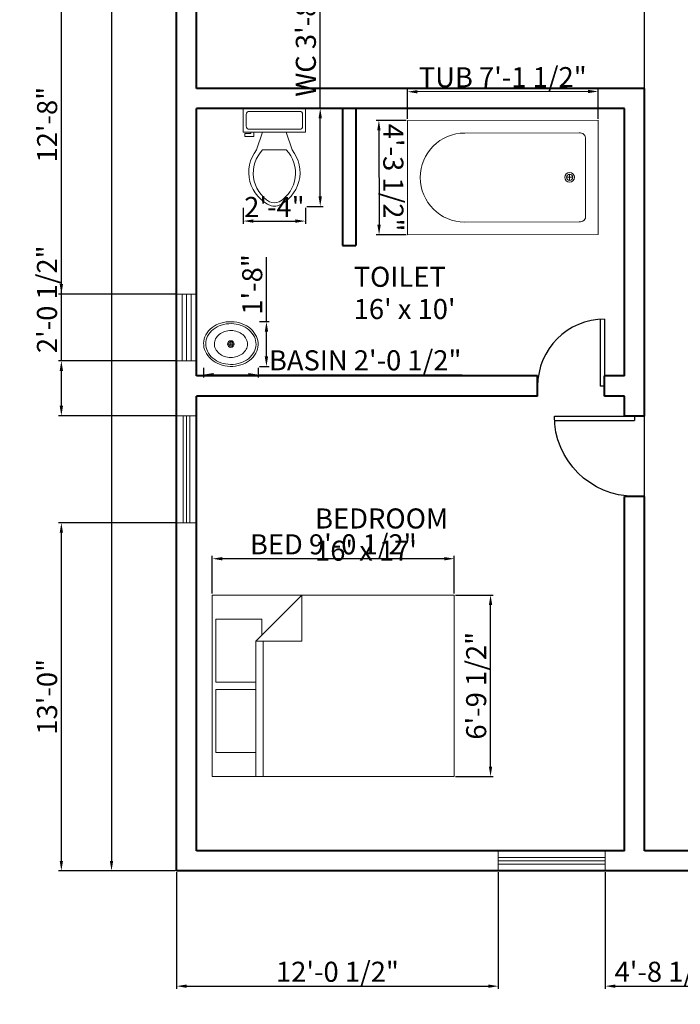
# Model space of a CAD drawing. Units: inches. Extents: x 2383 to 6214, y 970 to 3250.
# Tile 1 of 4: x 2383 to 2680, y 1059 to 1500. Entities that reach past the tile are written whole.
import ezdxf

# ---------------------------------------------------------------- set-up
doc = ezdxf.new("R2010")
doc.units = ezdxf.units.IN
for name, color, linetype, lineweight in [('A-ANNO-DIMS', 2, 'Continuous', 18), ('A-AREA-IDEN', 7, 'Continuous', 18), ('A-DOOR', 4, 'Continuous', 25), ('A-FLOR-FIXT', 8, 'Continuous', 18), ('A-FURN', 8, 'Continuous', 18), ('A-GLAZ', 4, 'Continuous', 18), ('A-WALL', 7, 'Continuous', 40)]:
    doc.layers.add(name, color=color, linetype=linetype, lineweight=lineweight)
doc.styles.get("Standard").update_dxf_attribs({"font": 'arial.ttf'})
doc.dimstyles.new('ISO-25', dxfattribs={"dimtxt": 9, "dimasz": 4.5, "dimexe": 1.25, "dimexo": 0.625, "dimtad": 1, "dimdec": 0, "dimlunit": 3, "dimtxsty": 'Standard', "dimcen": 2.5, "dimadec": 0, "dimazin": 0, "dimtfac": 1, "dimtdec": 0, "dimtmove": 0, "dimatfit": 3, "dimfxl": 1, "dimarcsym": 0})

# ---------------------------------------------------------------- blocks, each defined once
blk = doc.blocks.new('Toilet - top')
for p, q in [((9.5, -6), (9.5, -2)), ((-10, -8.5), (-8, -8.5)), ((-10, -9.5), (-10, -8.5)), ((-7, -9.5), (-10, -9.5)), ((-8, -8.5), (-8, -8)), ((-7, -8), (-7, -9.5)), ((-4, -8), (-6, -14)), ((4, -8), (6, -14)), ((4, -14), (-4, -14))]:
    blk.add_line(p, q)
blk.add_lwpolyline([(10.5, -8), (10.5, 0), (-10.5, 0), (-10.5, -8)], close=True)
for points in [[(-9.5, -2), (-9.5, -6)], [(8.5, -1), (-8.5, -1)], [(-8.5, -7), (8.5, -7)]]:
    blk.add_lwpolyline(points)
for centre, radius, start, end in [((-8.62, -1.88), 0.884, 81.8699, 188.1301), ((8.62, -1.88), 0.884, 351.8699, 98.1301), ((-8.62, -6.12), 0.884, 171.8699, 278.1301), ((8.62, -6.12), 0.884, 261.8699, 8.1301), ((3.52, -21.58), 12.17, 141.4691, 247.9714), ((4.2, -21.82), 11.33, 136.3677, 238.9468), ((-3.52, -21.58), 12.17, 292.0284, 38.5307), ((-4.2, -21.82), 11.33, 301.053, 43.6321), ((0, -27.88), 4, 245.7318, 294.2682), ((0, -29), 4, 254.8605, 285.1395)]:
    blk.add_arc(centre, radius, start, end)
blk = doc.blocks.new('Bed - Queen')
for p, q in [((0, -80.00003), (0, 0)), ((0, 0), (59.99999, 0)), ((59.99999, 0), (59.99999, -80.00003)), ((7.99999, -1.2), (28.79998, -1.2)), ((7.99999, -14.4), (7.99999, -1.2)), ((28.79998, -1.2), (28.79998, -14.4)), ((31.19999, -1.2), (51.99999, -1.2)), ((31.19999, -14.4), (31.19999, -1.2)), ((51.99999, -1.2), (51.99999, -16.4)), ((0, -14.4), (44.8, -14.4)), ((59.99999, -29.6), (44.8, -14.4)), ((44.8, -14.4), (44.8, -29.6)), ((44.8, -16.8), (0, -16.8)), ((51.99999, -16.4), (46.79936, -16.4)), ((44.8, -29.6), (59.99999, -29.6)), ((59.99999, -80.00003), (0, -80.00003))]:
    blk.add_line(p, q)
blk = doc.blocks.new('Bath Tub - 26 x 60 in.')
for p, q in [((8, -18), (10, -18)), ((9, -17), (9, -19))]:
    blk.add_line(p, q)
blk.add_lwpolyline([(0, -36), (0, 0), (60, 0), (60, -36)], close=True)
for points in [[(4, -30), (4, -6)], [(6, -4), (42, -4)], [(42, -32), (6, -32)]]:
    blk.add_lwpolyline(points)
for radius in [1.5, 1]:
    blk.add_circle((9, -18), radius)
for centre, radius, start, end in [((5.75, -5.75), 1.77, 81.8699, 188.1301), ((42, -18), 14, 270, 90), ((5.75, -30.25), 1.77, 171.8699, 278.1301)]:
    blk.add_arc(centre, radius, start, end)
blk = doc.blocks.new('Sink - Oval top')
for p, q in [((-1, 0), (1, 0)), ((0, 1), (0, -1))]:
    blk.add_line(p, q)
for points in [[(-12.23, 0.39, 0.117634), (-11.46, -3.36, 0.104469), (-8.88, -6.8, 0.090016), (-5.08, -9.07, 0.08192), (-0.32, -10.02, 0.08192), (4.49, -9.38, 0.090016), (8.42, -7.36, 0.104469), (11.22, -4.09, 0.117634), (12.23, -0.39, 0.117634), (11.46, 3.36, 0.104469), (8.88, 6.8, 0.090016), (5.08, 9.07, 0.08192), (0.32, 10.02, 0.08192), (-4.49, 9.38, 0.090016), (-8.42, 7.36, 0.104469), (-11.22, 4.09, 0.117634)], [(-11.29, 0.16, 0.118622), (-10.52, -3.25, 0.104678), (-8.07, -6.36, 0.089562), (-4.54, -8.37, 0.081185), (-0.13, -9.15, 0.081185), (4.3, -8.49, 0.089562), (7.89, -6.58, 0.104678), (10.42, -3.55, 0.118622), (11.29, -0.16, 0.118622), (10.52, 3.25, 0.104678), (8.07, 6.36, 0.089562), (4.54, 8.37, 0.081185), (0.13, 9.15, 0.081185), (-4.3, 8.49, 0.089562), (-7.89, 6.58, 0.104678), (-10.42, 3.55, 0.118622)], [(-7.42, 0.08, 0.118283), (-6.91, -2.17, 0.104607), (-5.29, -4.21, 0.089718), (-2.97, -5.53, 0.081436), (-0.07, -6.04, 0.081436), (2.84, -5.59, 0.089718), (5.2, -4.33, 0.104607), (6.86, -2.32, 0.118283), (7.42, -0.08, 0.118283), (6.91, 2.17, 0.104607), (5.29, 4.21, 0.089718), (2.97, 5.53, 0.081436), (0.07, 6.04, 0.081436), (-2.84, 5.59, 0.089718), (-5.2, 4.33, 0.104607), (-6.86, 2.32, 0.118283)]]:
    blk.add_lwpolyline(points, format="xyb", close=True)
for radius in [1.5, 1]:
    blk.add_circle((0, 0), radius)
blk = doc.blocks.new('*D16')
at = {"layer": 'A-ANNO-DIMS', "color": 0, "lineweight": -2, "transparency": 16777216}
for p, q in [((2453.2, 2078.68), (2423.38, 2078.68)), ((2424.63, 2074.18), (2424.63, 1123.18)), ((2453.2, 1118.68), (2423.38, 1118.68))]:
    blk.add_line(p, q, dxfattribs=at)
at = {"layer": 'A-ANNO-DIMS', "color": 0, "transparency": 16777216}
for points in [[(2423.88, 2074.18), (2425.38, 2074.18), (2424.63, 2078.68)], [(2423.88, 1123.18), (2425.38, 1123.18), (2424.63, 1118.68)]]:
    blk.add_solid(points, dxfattribs=at)
at = {"layer": 'Defpoints', "color": 0, "transparency": 16777216}
for p in [(2453.83, 2078.68), (2424.63, 1118.68), (2453.83, 1118.68)]:
    blk.add_point(p, dxfattribs=at)
at = {"layer": 'A-ANNO-DIMS', "color": 0, "transparency": 16777216, "insert": (2419.41, 1598.68), "char_height": 9, "attachment_point": 5, "rotation": 90}
blk.add_mtext("80'", dxfattribs=at)
blk = doc.blocks.new('DOOR-SWING-36IN')
for p, q in [((36, 36), (0, 36)), ((0, 36), (0, 34)), ((36, 34), (0, 34))]:
    blk.add_line(p, q)
blk.add_arc((0, 36), 36, 270, 0)
blk = doc.blocks.new('DOOR-SWING-30IN')
for p, q in [((28, 30), (28, 0)), ((30, 30), (30, 0)), ((30, 0), (28, 0))]:
    blk.add_line(p, q)
blk.add_arc((30, 0), 30, 90, 180)
blk = doc.blocks.new('WINDOW-48X9IN')
for p, q in [((3, 0), (3, 48)), ((4.5, 0), (4.5, 48)), ((6, 0), (6, 48))]:
    blk.add_line(p, q)
blk.add_lwpolyline([(0, 0), (0, 48), (9, 48), (9, 0)], close=True)
blk = doc.blocks.new('VENTILATOR-30X9IN')
for p, q in [((0, 0), (0, 30)), ((0, 30), (9, 30)), ((2.5, 0), (2.5, 30)), ((4.5, 0), (4.5, 30)), ((6.5, 0), (6.5, 30)), ((9, 30), (9, 0)), ((9, 0), (0, 0))]:
    blk.add_line(p, q)
blk = doc.blocks.new('*D29')
at = {"layer": 'A-ANNO-DIMS', "color": 0, "lineweight": -2, "transparency": 16777216}
for p, q in [((2469.84, 1243.05), (2469.84, 1259.96)), ((2573.91, 1258.71), (2474.34, 1258.71)), ((2578.41, 1243.05), (2578.41, 1259.96))]:
    blk.add_line(p, q, dxfattribs=at)
at = {"layer": 'A-ANNO-DIMS', "color": 0, "transparency": 16777216}
for points in [[(2474.34, 1259.46), (2474.34, 1257.96), (2469.84, 1258.71)], [(2573.91, 1259.46), (2573.91, 1257.96), (2578.41, 1258.71)]]:
    blk.add_solid(points, dxfattribs=at)
at = {"layer": 'Defpoints', "color": 0, "transparency": 16777216}
for p in [(2469.84, 1258.71), (2469.84, 1242.43), (2578.41, 1242.43)]:
    blk.add_point(p, dxfattribs=at)
at = {"layer": 'A-ANNO-DIMS', "color": 0, "transparency": 16777216, "insert": (2524.12, 1263.99), "char_height": 9, "attachment_point": 5}
blk.add_mtext('BED 9\'-0 1/2"', dxfattribs=at)
blk = doc.blocks.new('*D30')
at = {"layer": 'A-ANNO-DIMS', "color": 0, "lineweight": -2, "transparency": 16777216}
for p, q in [((2579.03, 1242.43), (2595.94, 1242.43)), ((2594.69, 1165.5), (2594.69, 1237.93)), ((2579.03, 1161), (2595.94, 1161))]:
    blk.add_line(p, q, dxfattribs=at)
at = {"layer": 'A-ANNO-DIMS', "color": 0, "transparency": 16777216}
for points in [[(2593.94, 1237.93), (2595.44, 1237.93), (2594.69, 1242.43)], [(2593.94, 1165.5), (2595.44, 1165.5), (2594.69, 1161)]]:
    blk.add_solid(points, dxfattribs=at)
at = {"layer": 'Defpoints', "color": 0, "transparency": 16777216}
for p in [(2578.41, 1242.43), (2594.69, 1242.43), (2578.41, 1161)]:
    blk.add_point(p, dxfattribs=at)
at = {"layer": 'A-ANNO-DIMS', "color": 0, "transparency": 16777216, "insert": (2589.41, 1201.72), "char_height": 9, "attachment_point": 5, "rotation": 90}
blk.add_mtext('6\'-9 1/2"', dxfattribs=at)
blk = doc.blocks.new('*D35')
at = {"layer": 'A-ANNO-DIMS', "color": 0, "lineweight": -2, "transparency": 16777216}
for p, q in [((2518.27, 1460.68), (2518.27, 1515.16)), ((2512.31, 1460.68), (2519.52, 1460.68)), ((2518.27, 1421.25), (2518.27, 1456.18)), ((2512.31, 1416.75), (2519.52, 1416.75))]:
    blk.add_line(p, q, dxfattribs=at)
at = {"layer": 'A-ANNO-DIMS', "color": 0, "transparency": 16777216}
for points in [[(2517.52, 1456.18), (2519.02, 1456.18), (2518.27, 1460.68)], [(2517.52, 1421.25), (2519.02, 1421.25), (2518.27, 1416.75)]]:
    blk.add_solid(points, dxfattribs=at)
at = {"layer": 'Defpoints', "color": 0, "transparency": 16777216}
for p in [(2511.68, 1460.68), (2518.27, 1460.68), (2511.68, 1416.75)]:
    blk.add_point(p, dxfattribs=at)
at = {"layer": 'A-ANNO-DIMS', "color": 0, "transparency": 16777216, "insert": (2512.99, 1490.17), "char_height": 9, "attachment_point": 5, "rotation": 90}
blk.add_mtext('WC 3\'-8"', dxfattribs=at)
blk = doc.blocks.new('*D36')
at = {"layer": 'A-ANNO-DIMS', "color": 0, "lineweight": -2, "transparency": 16777216}
for p, q in [((2483.77, 1416.13), (2483.77, 1408.91)), ((2511.68, 1416.13), (2511.68, 1408.91)), ((2488.27, 1410.16), (2507.18, 1410.16))]:
    blk.add_line(p, q, dxfattribs=at)
at = {"layer": 'A-ANNO-DIMS', "color": 0, "transparency": 16777216}
for points in [[(2488.27, 1410.91), (2488.27, 1409.41), (2483.77, 1410.16)], [(2507.18, 1410.91), (2507.18, 1409.41), (2511.68, 1410.16)]]:
    blk.add_solid(points, dxfattribs=at)
at = {"layer": 'Defpoints', "color": 0, "transparency": 16777216}
for p in [(2483.77, 1416.75), (2511.68, 1416.75), (2511.68, 1410.16)]:
    blk.add_point(p, dxfattribs=at)
at = {"layer": 'A-ANNO-DIMS', "color": 0, "transparency": 16777216, "insert": (2497.72, 1415.31), "char_height": 9, "attachment_point": 5}
blk.add_mtext('2\'-4"', dxfattribs=at)
blk = doc.blocks.new('*D39')
at = {"layer": 'A-ANNO-DIMS', "color": 0, "lineweight": -2, "transparency": 16777216}
for p, q in [((2557.42, 1455.95), (2557.4, 1469.41)), ((2638.45, 1468.29), (2561.9, 1468.17)), ((2642.97, 1456.09), (2642.95, 1469.55))]:
    blk.add_line(p, q, dxfattribs=at)
at = {"layer": 'A-ANNO-DIMS', "color": 0, "transparency": 16777216}
for points in [[(2561.9, 1468.92), (2561.9, 1467.42), (2557.4, 1468.16)], [(2638.45, 1469.04), (2638.45, 1467.54), (2642.95, 1468.3)]]:
    blk.add_solid(points, dxfattribs=at)
at = {"layer": 'Defpoints', "color": 0, "transparency": 16777216}
for p in [(2557.4, 1468.16), (2557.42, 1455.33), (2642.97, 1455.47)]:
    blk.add_point(p, dxfattribs=at)
at = {"layer": 'A-ANNO-DIMS', "color": 0, "transparency": 16777216, "insert": (2600.17, 1473.51), "char_height": 9, "attachment_point": 5, "rotation": 0.0956}
blk.add_mtext('TUB 7\'-1 1/2"', dxfattribs=at)
blk = doc.blocks.new('*D40')
at = {"layer": 'A-ANNO-DIMS', "color": 0, "lineweight": -2, "transparency": 16777216}
for p, q in [((2556.8, 1455.33), (2543.34, 1455.3)), ((2544.6, 1450.8), (2544.67, 1408.48)), ((2556.88, 1404), (2543.43, 1403.97))]:
    blk.add_line(p, q, dxfattribs=at)
at = {"layer": 'A-ANNO-DIMS', "color": 0, "transparency": 16777216}
for points in [[(2545.35, 1450.81), (2543.85, 1450.8), (2544.59, 1455.3)], [(2545.42, 1408.48), (2543.92, 1408.48), (2544.68, 1403.98)]]:
    blk.add_solid(points, dxfattribs=at)
at = {"layer": 'Defpoints', "color": 0, "transparency": 16777216}
for p in [(2557.42, 1455.33), (2544.68, 1403.98), (2557.51, 1404)]:
    blk.add_point(p, dxfattribs=at)
at = {"layer": 'A-ANNO-DIMS', "color": 0, "transparency": 16777216, "insert": (2549.91, 1429.65), "char_height": 9, "attachment_point": 5, "rotation": 270.0956}
blk.add_mtext('4\'-3 1/2"', dxfattribs=at)
blk = doc.blocks.new('*D51')
at = {"layer": 'A-ANNO-DIMS', "color": 0, "lineweight": -2, "transparency": 16777216}
for p, q in [((2465.91, 1344.31), (2465.91, 1340.01)), ((2490.46, 1344.31), (2490.46, 1340.01)), ((2470.41, 1341.26), (2485.96, 1341.26)), ((2490.46, 1341.26), (2581.93, 1341.26))]:
    blk.add_line(p, q, dxfattribs=at)
at = {"layer": 'A-ANNO-DIMS', "color": 0, "transparency": 16777216}
for points in [[(2470.41, 1342.01), (2470.41, 1340.51), (2465.91, 1341.26)], [(2485.96, 1342.01), (2485.96, 1340.51), (2490.46, 1341.26)]]:
    blk.add_solid(points, dxfattribs=at)
at = {"layer": 'Defpoints', "color": 0, "transparency": 16777216}
for p in [(2465.91, 1344.94), (2490.46, 1344.94), (2490.46, 1341.26)]:
    blk.add_point(p, dxfattribs=at)
at = {"layer": 'A-ANNO-DIMS', "color": 0, "transparency": 16777216, "insert": (2538.45, 1346.53), "char_height": 9, "attachment_point": 5}
blk.add_mtext('BASIN 2\'-0 1/2"', dxfattribs=at)
blk = doc.blocks.new('*D52')
at = {"layer": 'A-ANNO-DIMS', "color": 0, "lineweight": -2, "transparency": 16777216}
for p, q in [((2494.14, 1365.07), (2494.14, 1393.9)), ((2491.09, 1365.07), (2495.39, 1365.07)), ((2494.14, 1349.44), (2494.14, 1360.57)), ((2491.09, 1344.94), (2495.39, 1344.94))]:
    blk.add_line(p, q, dxfattribs=at)
at = {"layer": 'A-ANNO-DIMS', "color": 0, "transparency": 16777216}
for points in [[(2493.39, 1360.57), (2494.89, 1360.57), (2494.14, 1365.07)], [(2493.39, 1349.44), (2494.89, 1349.44), (2494.14, 1344.94)]]:
    blk.add_solid(points, dxfattribs=at)
at = {"layer": 'Defpoints', "color": 0, "transparency": 16777216}
for p in [(2490.46, 1365.07), (2494.14, 1365.07), (2490.46, 1344.94)]:
    blk.add_point(p, dxfattribs=at)
at = {"layer": 'A-ANNO-DIMS', "color": 0, "transparency": 16777216, "insert": (2488.92, 1381.74), "char_height": 9, "attachment_point": 5, "rotation": 90}
blk.add_mtext('1\'-8"', dxfattribs=at)
blk = doc.blocks.new('*D53')
at = {"layer": 'A-ANNO-DIMS', "color": 0, "lineweight": -2, "transparency": 16777216}
for p, q in [((2453.83, 1118.05), (2453.83, 1065.73)), ((2598.17, 1118.05), (2598.17, 1065.73)), ((2458.33, 1066.98), (2593.67, 1066.98))]:
    blk.add_line(p, q, dxfattribs=at)
at = {"layer": 'A-ANNO-DIMS', "color": 0, "transparency": 16777216}
for points in [[(2458.33, 1067.73), (2458.33, 1066.23), (2453.83, 1066.98)], [(2593.67, 1067.73), (2593.67, 1066.23), (2598.17, 1066.98)]]:
    blk.add_solid(points, dxfattribs=at)
at = {"layer": 'Defpoints', "color": 0, "transparency": 16777216}
for p in [(2453.83, 1118.68), (2598.17, 1118.68), (2598.17, 1066.98)]:
    blk.add_point(p, dxfattribs=at)
at = {"layer": 'A-ANNO-DIMS', "color": 0, "transparency": 16777216, "insert": (2526, 1072.26), "char_height": 9, "attachment_point": 5}
blk.add_mtext('12\'-0 1/2"', dxfattribs=at)
blk = doc.blocks.new('*D54')
at = {"layer": 'A-ANNO-DIMS', "color": 0, "lineweight": -2, "transparency": 16777216}
for p, q in [((2646.17, 1118.05), (2646.17, 1065.73)), ((2702.83, 1118.05), (2702.83, 1065.73)), ((2650.67, 1066.98), (2698.33, 1066.98))]:
    blk.add_line(p, q, dxfattribs=at)
at = {"layer": 'A-ANNO-DIMS', "color": 0, "transparency": 16777216}
for points in [[(2650.67, 1067.73), (2650.67, 1066.23), (2646.17, 1066.98)], [(2698.33, 1067.73), (2698.33, 1066.23), (2702.83, 1066.98)]]:
    blk.add_solid(points, dxfattribs=at)
at = {"layer": 'Defpoints', "color": 0, "transparency": 16777216}
for p in [(2646.17, 1118.68), (2702.83, 1118.68), (2702.83, 1066.98)]:
    blk.add_point(p, dxfattribs=at)
at = {"layer": 'A-ANNO-DIMS', "color": 0, "transparency": 16777216, "insert": (2674.5, 1072.26), "char_height": 9, "attachment_point": 5}
blk.add_mtext('4\'-8 1/2"', dxfattribs=at)
blk = doc.blocks.new('*D56')
at = {"layer": 'A-ANNO-DIMS', "color": 0, "lineweight": -2, "transparency": 16777216}
for p, q in [((2663.83, 1128.3), (2663.83, 2131.63)), ((2668.33, 2130.38), (2779.33, 2130.38)), ((2783.83, 1128.3), (2783.83, 2131.63))]:
    blk.add_line(p, q, dxfattribs=at)
at = {"layer": 'A-ANNO-DIMS', "color": 0, "transparency": 16777216}
for points in [[(2668.33, 2131.13), (2668.33, 2129.63), (2663.83, 2130.38)], [(2779.33, 2131.13), (2779.33, 2129.63), (2783.83, 2130.38)]]:
    blk.add_solid(points, dxfattribs=at)
at = {"layer": 'Defpoints', "color": 0, "transparency": 16777216}
for p in [(2783.83, 2130.38), (2663.83, 1127.68), (2783.83, 1127.68)]:
    blk.add_point(p, dxfattribs=at)
at = {"layer": 'A-ANNO-DIMS', "color": 0, "transparency": 16777216, "insert": (2723.83, 2135.6), "char_height": 9, "attachment_point": 5}
blk.add_mtext('10\'-0"', dxfattribs=at)
blk = doc.blocks.new('*D59')
at = {"layer": 'A-ANNO-DIMS', "color": 0, "lineweight": -2, "transparency": 16777216}
for p, q in [((2453.2, 1274.85), (2400.88, 1274.85)), ((2402.13, 1123.18), (2402.13, 1270.35)), ((2453.2, 1118.68), (2400.88, 1118.68))]:
    blk.add_line(p, q, dxfattribs=at)
at = {"layer": 'A-ANNO-DIMS', "color": 0, "transparency": 16777216}
for points in [[(2401.38, 1270.35), (2402.88, 1270.35), (2402.13, 1274.85)], [(2401.38, 1123.18), (2402.88, 1123.18), (2402.13, 1118.68)]]:
    blk.add_solid(points, dxfattribs=at)
at = {"layer": 'Defpoints', "color": 0, "transparency": 16777216}
for p in [(2402.13, 1274.85), (2453.83, 1274.85), (2453.83, 1118.68)]:
    blk.add_point(p, dxfattribs=at)
at = {"layer": 'A-ANNO-DIMS', "color": 0, "transparency": 16777216, "insert": (2396.9, 1196.77), "char_height": 9, "attachment_point": 5, "rotation": 90}
blk.add_mtext('13\'-0"', dxfattribs=at)
blk = doc.blocks.new('*D60')
at = {"layer": 'A-ANNO-DIMS', "color": 0, "lineweight": -2, "transparency": 16777216}
for p, q in [((2402.13, 1347.43), (2402.13, 1398.23)), ((2453.2, 1347.43), (2400.88, 1347.43)), ((2402.13, 1327.35), (2402.13, 1342.93)), ((2453.2, 1322.85), (2400.88, 1322.85))]:
    blk.add_line(p, q, dxfattribs=at)
at = {"layer": 'A-ANNO-DIMS', "color": 0, "transparency": 16777216}
for points in [[(2401.38, 1342.93), (2402.88, 1342.93), (2402.13, 1347.43)], [(2401.38, 1327.35), (2402.88, 1327.35), (2402.13, 1322.85)]]:
    blk.add_solid(points, dxfattribs=at)
at = {"layer": 'Defpoints', "color": 0, "transparency": 16777216}
for p in [(2402.13, 1347.43), (2453.83, 1347.43), (2453.83, 1322.85)]:
    blk.add_point(p, dxfattribs=at)
at = {"layer": 'A-ANNO-DIMS', "color": 0, "transparency": 16777216, "insert": (2396.85, 1375.08), "char_height": 9, "attachment_point": 5, "rotation": 90}
blk.add_mtext('2\'-0 1/2"', dxfattribs=at)
blk = doc.blocks.new('*D61')
at = {"layer": 'A-ANNO-DIMS', "color": 0, "lineweight": -2, "transparency": 16777216}
for p, q in [((2453.2, 1529.36), (2400.88, 1529.36)), ((2402.13, 1381.93), (2402.13, 1524.86)), ((2453.2, 1377.43), (2400.88, 1377.43))]:
    blk.add_line(p, q, dxfattribs=at)
at = {"layer": 'A-ANNO-DIMS', "color": 0, "transparency": 16777216}
for points in [[(2401.38, 1524.86), (2402.88, 1524.86), (2402.13, 1529.36)], [(2401.38, 1381.93), (2402.88, 1381.93), (2402.13, 1377.43)]]:
    blk.add_solid(points, dxfattribs=at)
at = {"layer": 'Defpoints', "color": 0, "transparency": 16777216}
for p in [(2402.13, 1529.36), (2453.83, 1529.36), (2453.83, 1377.43)]:
    blk.add_point(p, dxfattribs=at)
at = {"layer": 'A-ANNO-DIMS', "color": 0, "transparency": 16777216, "insert": (2396.91, 1453.4), "char_height": 9, "attachment_point": 5, "rotation": 90}
blk.add_mtext('12\'-8"', dxfattribs=at)

msp = doc.modelspace()

# ---------------------------------------------------------------- linework, layer by layer
at = {"layer": 'A-WALL'}
for p, q in [((2453.83, 1118.68), (2453.83, 2078.68)), ((2462.83, 1469.68), (2462.83, 1616.68)), ((2663.83, 1469.68), (2462.83, 1469.68)), ((2663.83, 1322.68), (2663.83, 1469.68)), ((2654.83, 1460.68), (2462.83, 1460.68)), ((2462.83, 1340.68), (2462.83, 1460.68)), ((2528.32, 1460.68), (2528.32, 1399.26)), ((2534.32, 1460.68), (2534.32, 1399.26)), ((2654.83, 1340.68), (2654.83, 1460.68)), ((2528.32, 1399.26), (2534.32, 1399.26)), ((2615.83, 1340.68), (2462.83, 1340.68)), ((2615.83, 1331.68), (2615.83, 1340.68)), ((2654.83, 1340.68), (2645.83, 1340.68)), ((2645.83, 1331.68), (2645.83, 1340.68)), ((2462.83, 1127.68), (2462.83, 1331.68)), ((2615.83, 1331.68), (2462.83, 1331.68)), ((2654.83, 1331.68), (2645.83, 1331.68)), ((2654.83, 1322.68), (2654.83, 1331.68)), ((2663.83, 1322.68), (2654.83, 1322.68)), ((2654.83, 1127.68), (2654.83, 1286.68)), ((2663.83, 1286.68), (2654.83, 1286.68)), ((2663.83, 1127.68), (2663.83, 1286.68)), ((2654.83, 1127.68), (2462.83, 1127.68)), ((2702.83, 1127.68), (2663.83, 1127.68)), ((2702.83, 1118.68), (2453.83, 1118.68))]:
    msp.add_line(p, q, dxfattribs=at)

# ---------------------------------------------------------------- block references
at = {"layer": 'A-DOOR'}
msp.add_blockref('DOOR-SWING-30IN', (2615.83, 1336.18), dxfattribs=at)
at = {"layer": 'A-DOOR', "extrusion": (0, 0, -1), "zscale": -1}
msp.add_blockref('DOOR-SWING-36IN', (-2659.33, 1286.68), dxfattribs=at)
at = {"layer": 'A-FLOR-FIXT', "xscale": 1.329298306698029, "yscale": 1.329298306698029, "zscale": 1.329298306698029}
msp.add_blockref('Toilet - top', (2497.72, 1460.68), dxfattribs=at)
at = {"layer": 'A-FLOR-FIXT', "xscale": 1.425793959532678, "yscale": 1.425793959532678, "zscale": 1.425793959532678, "rotation": 180.0955849895595}
msp.add_blockref('Bath Tub - 26 x 60 in.', (2643.05, 1404.14), dxfattribs=at)
at = {"layer": 'A-FLOR-FIXT'}
msp.add_blockref('Sink - Oval top', (2478.19, 1355.01), dxfattribs=at)
at = {"layer": 'A-FURN', "xscale": 1.357085414550351, "yscale": 1.357085414550351, "zscale": 1.357085414550351, "rotation": 90}
msp.add_blockref('Bed - Queen', (2469.84, 1161), dxfattribs=at)
at = {"layer": 'A-GLAZ'}
for name, p in [('VENTILATOR-30X9IN', (2453.83, 1347.43)), ('WINDOW-48X9IN', (2453.83, 1274.85))]:
    msp.add_blockref(name, p, dxfattribs=at)
at = {"layer": 'A-GLAZ', "rotation": 270.0000000000005}
msp.add_blockref('WINDOW-48X9IN', (2598.18, 1127.68), dxfattribs=at)

# ---------------------------------------------------------------- texts
at = {"layer": 'A-AREA-IDEN'}
for s, p in [('TOILET', (2533.29, 1380.67)), ("16' x 10'", (2533.29, 1366.21)), ('BEDROOM ', (2515.96, 1272.26)), ("16' x 17'", (2515.96, 1257.81))]:
    msp.add_text(s, height=9, dxfattribs=at).set_placement(p)

# ---------------------------------------------------------------- dimensions: what is measured, and where the dimension line sits
at = {"layer": 'A-ANNO-DIMS'}
for base, p1, p2, picture, middle in [((2783.83, 2130.38), (2663.83, 1127.68), (2783.83, 1127.68), '*D56', (2723.83, 2135.6)), ((2511.68, 1410.16), (2483.77, 1416.75), (2511.68, 1416.75), '*D36', (2497.72, 1415.31)), ((2598.17, 1066.98), (2453.83, 1118.68), (2598.17, 1118.68), '*D53', (2526, 1072.26)), ((2702.83, 1066.98), (2646.17, 1118.68), (2702.83, 1118.68), '*D54', (2674.5, 1072.26))]:
    dim = msp.add_linear_dim(base=base, p1=p1, p2=p2, dimstyle='ISO-25', override={"dimdec": 1, "dimlfac": 1, "dimrnd": 0, "dimzin": 1, "dimdsep": 46, "dimlunit": 4, "dimfrac": 2}, dxfattribs=at)
    dim.commit()
    dim.dimension.update_dxf_attribs({"geometry": picture, "text_midpoint": middle})
for base, p1, p2, angle, override, picture, middle in [((2424.63, 1118.68), (2453.83, 2078.68), (2453.83, 1118.68), 90, {"dimclrd": 0, "dimclre": 0, "dimclrt": 0}, '*D16', (2419.41, 1598.68)), ((2402.13, 1529.36), (2453.83, 1377.43), (2453.83, 1529.36), 90, {"dimdec": 1, "dimlfac": 1, "dimrnd": 0, "dimzin": 1, "dimdsep": 46, "dimlunit": 4, "dimfrac": 2}, '*D61', (2396.91, 1453.4)), ((2544.68, 1403.98), (2557.42, 1455.33), (2557.51, 1404), 270.0956, {"dimdec": 1, "dimlfac": 1, "dimrnd": 0, "dimzin": 1, "dimdsep": 46, "dimlunit": 4, "dimfrac": 2}, '*D40', (2549.91, 1429.65)), ((2402.13, 1347.43), (2453.83, 1322.85), (2453.83, 1347.43), 90, {"dimdec": 1, "dimlfac": 1, "dimrnd": 0, "dimzin": 1, "dimdsep": 46, "dimlunit": 4, "dimfrac": 2}, '*D60', (2396.85, 1375.08)), ((2494.14, 1365.07), (2490.46, 1344.94), (2490.46, 1365.07), 90, {"dimdec": 1, "dimlfac": 1, "dimrnd": 0, "dimzin": 1, "dimdsep": 46, "dimlunit": 4, "dimfrac": 2}, '*D52', (2488.92, 1381.74)), ((2402.13, 1274.85), (2453.83, 1118.68), (2453.83, 1274.85), 90, {"dimdec": 1, "dimlfac": 1, "dimrnd": 0, "dimzin": 1, "dimdsep": 46, "dimlunit": 4, "dimfrac": 2}, '*D59', (2396.9, 1196.77)), ((2594.69, 1242.43), (2578.41, 1161), (2578.41, 1242.43), 90, {"dimdec": 1, "dimlfac": 1, "dimrnd": 0, "dimzin": 1, "dimdsep": 46, "dimlunit": 4, "dimfrac": 2}, '*D30', (2589.41, 1201.72))]:
    dim = msp.add_linear_dim(base=base, p1=p1, p2=p2, angle=angle, dimstyle='ISO-25', override=override, dxfattribs=at)
    dim.commit()
    dim.dimension.update_dxf_attribs({"geometry": picture, "text_midpoint": middle})
for base, p1, p2, angle, text, picture, middle in [((2518.27, 1460.68), (2511.68, 1416.75), (2511.68, 1460.68), 90, 'WC <>', '*D35', (2512.99, 1490.17)), ((2557.4003, 1468.1583), (2642.9693, 1455.4689), (2557.4217, 1455.3262), 180.0956, 'TUB <>', '*D39', (2600.1653, 1473.5082)), ((2469.84, 1258.71), (2578.41, 1242.43), (2469.84, 1242.43), 180, 'BED <>', '*D29', (2524.12, 1263.99))]:
    dim = msp.add_linear_dim(base=base, p1=p1, p2=p2, angle=angle, text=text, dimstyle='ISO-25', override={"dimdec": 1, "dimlfac": 1, "dimrnd": 0, "dimzin": 1, "dimdsep": 46, "dimlunit": 4, "dimfrac": 2}, dxfattribs=at)
    dim.commit()
    dim.dimension.update_dxf_attribs({"geometry": picture, "text_midpoint": middle})
dim = msp.add_linear_dim(base=(2490.4606, 1341.255), p1=(2465.9097, 1344.9376), p2=(2490.4606, 1344.9376), text='BASIN <>', dimstyle='ISO-25', override={"dimdec": 1, "dimlfac": 1, "dimrnd": 0, "dimzin": 1, "dimdsep": 46, "dimlunit": 4, "dimfrac": 2}, dxfattribs=at)
dim.commit()
dim.dimension.update_dxf_attribs({"geometry": '*D51', "text_midpoint": (2538.4461, 1346.5335)})

doc.saveas('drawing.dxf')
